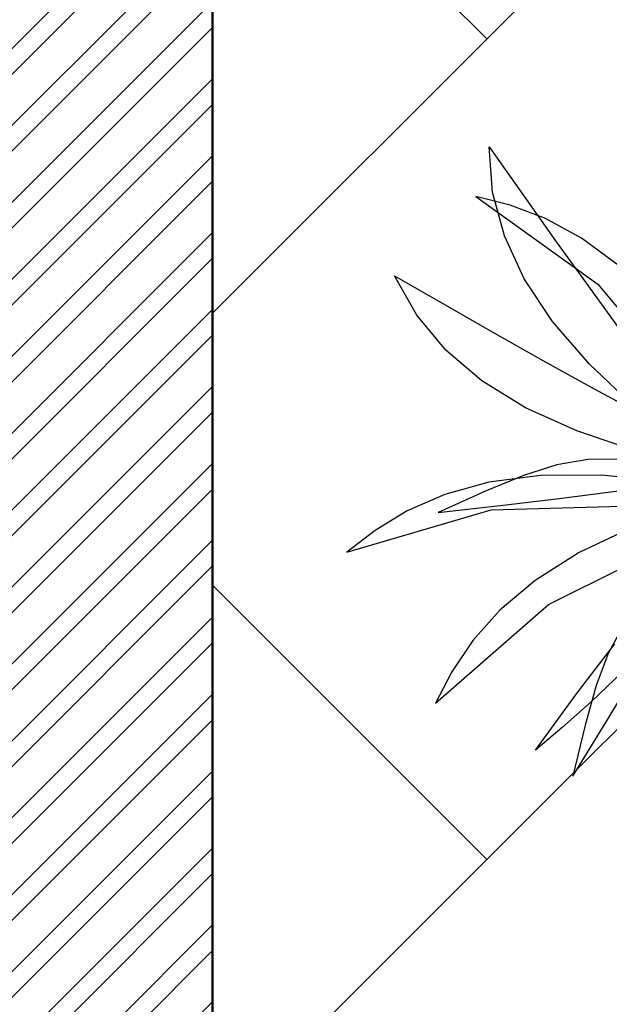
# Model space of a CAD drawing. Units: inches. Extents: x 3590 to 5167, y 65 to 1917.
# Tile 49 of 100: x 4927 to 4947, y 1504 to 1538. Entities that reach past the tile are written whole.
import ezdxf

# ---------------------------------------------------------------- set-up
doc = ezdxf.new("R2010")
doc.units = ezdxf.units.IN
for name, color, linetype, lineweight in [('A-FLOR-PATT', 8, 'Continuous', 13), ('A-WALL', 7, 'Continuous', 50), ('A-WALL-PATT', 251, 'Continuous', 13), ('L-PLNT', 94, 'Continuous', 18)]:
    doc.layers.add(name, color=color, linetype=linetype, lineweight=lineweight)
doc.layers.add('DIENHOA', color=3, linetype='Continuous')

# ---------------------------------------------------------------- blocks, each defined once
blk = doc.blocks.new('Cay03_mb')
at = {"layer": 'DIENHOA'}
for p, q in [((-365.2, 390.3), (-414.4, 402.8)), ((-414.4, 402.8), (-240.2, 277.8)), ((-314.9, 371.3), (-365.2, 390.3)), ((-263.5, 343.5), (-314.9, 371.3)), ((-211.2, 304.6), (-263.5, 343.5)), ((-240.2, 277.8), (-88.4, 94.9)), ((-298.6, 20.1), (-345, 5.4)), ((-254.7, 27.4), (-298.6, 20.1)), ((-208, 27.8), (-254.7, 27.4)), ((-345, 5.4), (-399.6, -17.1)), ((-225.8, -18.9), (-165.8, -11.3)), ((-399.6, -17.1), (-468, -47.9)), ((-375.6, -37.8), (-295.3, -27.9)), ((-295.3, -27.9), (-225.8, -18.9)), ((-468, -47.9), (-375.6, -37.8)), ((-271, -306.6), (-216.3, -235.6)), ((-206.3, -276.5), (-249.6, -317.8)), ((-329.5, -387.1), (-271, -306.6)), ((-249.6, -317.8), (-291, -354.7)), ((-291, -354.7), (-329.5, -387.1))]:
    blk.add_line(p, q, dxfattribs=at)
for points in [[(-395.6, 473.7), (-347.5, 405.6), (-300.6, 339.5), (-254.3, 275.1), (-208.3, 212.3), (-161.9, 150.9), (-114.8, 90.7), (-66.5, 31.6), (-16.4, -26.7)], [(-16.4, -26.7), (-108.3, 38.6), (-186.9, 101.7), (-252.4, 163.5), (-305.1, 224.4), (-345.4, 285.2), (-373.7, 346.6), (-390.4, 409.2), (-395.6, 473.7)], [(-530.5, 289.7), (-458.3, 248.1), (-387.9, 207.8), (-318.9, 168.7), (-250.8, 131.1), (-182.9, 94.8), (-114.9, 59.9), (-46.2, 26.5), (23.7, -5.4)], [(23.7, -5.4), (-87.2, 15.2), (-185, 39.6), (-270.3, 68.2), (-343.7, 101.4), (-405.9, 139.7), (-457.3, 183.5), (-498.7, 233.4), (-530.5, 289.7)], [(-16.4, -26.7), (-134, -4.7), (-235.3, 5.3), (-322, 4.7), (-395.9, -5), (-458.7, -22.3), (-512.3, -45.7), (-558.2, -73.6), (-598.4, -104.7)], [(-471.9, -320.3), (-310.5, -179.3), (-97.7, -73.3), (23.7, -5.4)], [(23.7, -5.4), (-92.3, -34.8), (-188.4, -68.2), (-266.9, -105.1), (-329.9, -144.9), (-379.7, -187), (-418.5, -230.7), (-448.5, -275.3), (-471.9, -320.3)], [(-598.4, -104.7), (-392.7, -44.4), (-155, -37.4), (-16.4, -26.7)], [(-276.2, -424.4), (-227.3, -345.4), (-185.7, -276.1), (-150, -215.7), (-119.1, -163.8), (-91.5, -119.5), (-66, -82.3), (-41.4, -51.6), (-16.4, -26.7)], [(-16.4, -26.7), (-84.9, -86), (-137, -133.1), (-175.8, -173), (-204.3, -210), (-225.5, -249.1), (-242.5, -294.7), (-258.4, -351.6), (-276.2, -424.4)]]:
    blk.add_lwpolyline(points, dxfattribs=at)

msp = doc.modelspace()

# ---------------------------------------------------------------- hatches: boundary and pattern name
at = {"layer": 'A-FLOR-PATT', "transparency": 33554687}
h = msp.add_hatch(dxfattribs=at)
h.set_pattern_fill('AR-HBONE', color=256, scale=0.2)
h.set_pattern_definition([(45, (-588.972, 0), (0, 28.73682), [60.96, -20.32]), (135, (-574.604, 14.368), (3e-15, 28.73682), [60.96, -20.32])])
h.paths.add_polyline_path([(5071.274, 1796.999), (4933.274, 1796.999), (4933.274, 1753.999), (4962.774, 1753.999, -0.414214), (4928.774, 1719.999), (4933.274, 1718.999), (4933.274, 1334.999), (5071.274, 1334.999)])
h.paths.add_polyline_path([(4951.78, 1521.077), (4951.715, 1521.04), (4951.563, 1520.895)], flags=16)
h.paths.add_polyline_path([(4952.267, 1521.376), (4952.198, 1521.371), (4952.198, 1521.356)], flags=0)
h.paths.add_polyline_path([(4967.051, 1529.728), (4965.231, 1528.694), (4963.411, 1527.714), (4961.756, 1526.851), (4963.589, 1527.449), (4964.036, 1527.478), (4962.975, 1527.249), (4961.76, 1526.852), (4959.792, 1525.834), (4958.005, 1524.895), (4956.24, 1523.93), (4954.504, 1522.919), (4954.129, 1522.682), (4953.361, 1521.997), (4953.366, 1521.998), (4953.605, 1522.064), (4955.106, 1522.761), (4956.921, 1523.434), (4958.678, 1523.915), (4960.358, 1524.2), (4961.945, 1524.286), (4964.171, 1524.108), (4965.958, 1523.309), (4963.863, 1522.976), (4965.187, 1522.499), (4963.366, 1522.497), (4961.545, 1522.487), (4959.764, 1522.461), (4958.304, 1522.419), (4957.974, 1522.388), (4956.307, 1522.232), (4954.718, 1522.071), (4953.251, 1521.899), (4953.525, 1521.623), (4954.331, 1521.379), (4956.243, 1521.23), (4958.039, 1520.93), (4959.684, 1520.483), (4961.16, 1519.896), (4963.107, 1518.8), (4964.393, 1517.325), (4962.973, 1517.726), (4964.558, 1516.661), (4965.407, 1515.708), (4963.507, 1516.322), (4961.68, 1517.005), (4959.935, 1517.745), (4958.282, 1518.528), (4956.732, 1519.343), (4955.295, 1520.175), (4954.672, 1520.572), (4954.513, 1520.627), (4955.658, 1519.318), (4956.703, 1517.982), (4957.644, 1516.647), (4958.485, 1515.334), (4959.55, 1513.524), (4960.438, 1511.769), (4958.841, 1513.62), (4957.452, 1515.325), (4955.819, 1517.459), (4956.665, 1515.448), (4957.111, 1513.923), (4957.447, 1511.714), (4957.076, 1509.793), (4956.538, 1511.11), (4955.992, 1512.569), (4955.444, 1514.125), (4954.898, 1515.735), (4954.357, 1517.356), (4953.824, 1518.943), (4953.305, 1520.452), (4953.065, 1521.116), (4952.971, 1521.146), (4952.949, 1521.086), (4952.73, 1520.199), (4953.37, 1518.024), (4953.757, 1516.373), (4954.051, 1514.765), (4954.264, 1513.221), (4954.471, 1511.131), (4954.497, 1510.402), (4954.409, 1511.76), (4954.264, 1513.221), (4954.051, 1514.765), (4953.757, 1516.373), (4953.37, 1518.024), (4952.877, 1519.698), (4952.716, 1520.141), (4952.533, 1519.059), (4952.374, 1517.789), (4952.219, 1516.312), (4952.046, 1514.6), (4951.833, 1512.626), (4951.557, 1510.363), (4951.203, 1512.168), (4950.852, 1514.339), (4950.985, 1516.376), (4951.66, 1518.286), (4952.593, 1520.481), (4952.357, 1521.13), (4951.855, 1520.328), (4950.839, 1518.908), (4949.777, 1517.587), (4948.916, 1516.617), (4948.111, 1515.256), (4947.089, 1513.554), (4945.889, 1511.615), (4946.326, 1513.402), (4946.562, 1514.249), (4945.528, 1513.327), (4944.581, 1512.531), (4946.018, 1514.508), (4947.204, 1516.048), (4947.893, 1517.313), (4949.307, 1518.764), (4950.414, 1519.767), (4950.451, 1519.806), (4952.267, 1521.376), (4951.645, 1521.493), (4950.404, 1521.18), (4948.044, 1520.359), (4946.119, 1519.452), (4944.572, 1518.475), (4943.35, 1517.443), (4941.997, 1515.92), (4941.661, 1515.275), (4942.813, 1516.99), (4944.572, 1518.475), (4946.119, 1519.452), (4948.044, 1520.359), (4950.404, 1521.18), (4951.645, 1521.493), (4949.647, 1521.868), (4948.6, 1521.756), (4947.126, 1521.57), (4945.42, 1521.348), (4943.45, 1521.105), (4941.183, 1520.856), (4942.86, 1521.613), (4943.873, 1522.03), (4942.952, 1521.909), (4941.41, 1521.485), (4939.543, 1520.67), (4938.968, 1520.226), (4940.733, 1521.299), (4942.952, 1521.909), (4943.702, 1522.008), (4945.894, 1522.7), (4947.565, 1522.714), (4948.921, 1522.566), (4951.131, 1522.183), (4950.971, 1522.297), (4948.129, 1523.006), (4946.035, 1523.707), (4944.232, 1524.521), (4942.707, 1525.461), (4941.444, 1526.537), (4940.43, 1527.761), (4939.649, 1529.143), (4941.421, 1528.122), (4943.147, 1527.132), (4944.841, 1526.175), (4946.514, 1525.25), (4948.179, 1524.359), (4948.365, 1524.263), (4946.475, 1526.045), (4945.181, 1527.54), (4944.19, 1529.033), (4943.496, 1530.54), (4943.278, 1531.36), (4942.498, 1531.919), (4943.114, 1531.762), (4942.959, 1533.659), (4944.14, 1531.989), (4944.612, 1531.323), (4946.202, 1530.463), (4947.486, 1529.509), (4948.79, 1528.226), (4950.368, 1526.237), (4949.485, 1528.155), (4948.851, 1530.123), (4948.491, 1532.041), (4948.381, 1533.918), (4948.501, 1535.76), (4948.827, 1537.573), (4949.418, 1535.565), (4949.957, 1533.569), (4950.464, 1531.586), (4950.961, 1529.617), (4951.391, 1527.954), (4951.724, 1530.687), (4952.201, 1532.58), (4952.889, 1534.33), (4953.77, 1535.951), (4954.827, 1537.46), (4954.521, 1535.39), (4954.273, 1533.937), (4955.58, 1535.663), (4956.748, 1536.739), (4956.159, 1534.78), (4955.589, 1532.873), (4955.043, 1531.006), (4954.525, 1529.166), (4954.038, 1527.341), (4953.638, 1525.733), (4953.611, 1525.586), (4953.398, 1524.166), (4953.382, 1524.009), (4954.07, 1525.476), (4954.912, 1527.022), (4956.136, 1528.894), (4957.847, 1530.577), (4959.376, 1531.54), (4958.256, 1530.104), (4957.143, 1528.663), (4956.066, 1527.243), (4955.056, 1525.871), (4954.141, 1524.571), (4953.352, 1523.372), (4953.311, 1523.303), (4953.273, 1522.925), (4953.261, 1522.382), (4954.103, 1523.373), (4954.63, 1524.284), (4955.961, 1526.358), (4957.23, 1528.13), (4958.421, 1529.609), (4960.037, 1531.368), (4961.374, 1532.375), (4962.101, 1532.77), (4961.07, 1531.061), (4959.987, 1529.438), (4958.869, 1527.908), (4958.15, 1527.007), (4959.803, 1528.003), (4961.589, 1528.793), (4963.391, 1529.328), (4965.211, 1529.632)], flags=16)
h.paths.add_polyline_path([(4962.944, 1523.182), (4961.107, 1523.422), (4960.392, 1523.362), (4962.35, 1523.331)], flags=0)
h.paths.add_polyline_path([(5049.541, 1584.551), (5049.476, 1584.515), (5049.325, 1584.37)], flags=16)
h.paths.add_polyline_path([(5050.028, 1584.851), (5049.959, 1584.845), (5049.959, 1584.83)], flags=0)
h.paths.add_polyline_path([(5042.333, 1581.949), (5043.88, 1582.926), (5045.806, 1583.833), (5048.165, 1584.654), (5049.406, 1584.967), (5047.408, 1585.342), (5046.361, 1585.231), (5044.888, 1585.044), (5043.181, 1584.822), (5041.211, 1584.579), (5038.944, 1584.33), (5040.622, 1585.087), (5041.634, 1585.504), (5040.713, 1585.383), (5039.171, 1584.959), (5037.304, 1584.144), (5036.729, 1583.7), (5038.494, 1584.773), (5040.713, 1585.383), (5041.463, 1585.482), (5043.655, 1586.174), (5045.326, 1586.188), (5046.682, 1586.04), (5048.893, 1585.657), (5048.732, 1585.771), (5045.891, 1586.48), (5043.796, 1587.181), (5041.994, 1587.996), (5040.468, 1588.935), (5039.205, 1590.011), (5038.191, 1591.235), (5037.41, 1592.617), (5039.182, 1591.596), (5040.909, 1590.607), (5042.602, 1589.649), (5044.275, 1588.724), (5045.94, 1587.833), (5046.126, 1587.738), (5044.237, 1589.519), (5042.942, 1591.015), (5041.952, 1592.508), (5041.257, 1594.014), (5041.039, 1594.834), (5040.26, 1595.393), (5040.875, 1595.237), (5040.721, 1597.133), (5041.901, 1595.463), (5042.373, 1594.798), (5043.963, 1593.938), (5045.247, 1592.983), (5046.552, 1591.701), (5048.129, 1589.712), (5047.247, 1591.63), (5046.613, 1593.597), (5046.252, 1595.515), (5046.142, 1597.392), (5046.262, 1599.234), (5046.588, 1601.047), (5047.179, 1599.039), (5047.718, 1597.043), (5048.225, 1595.06), (5048.722, 1593.091), (5049.152, 1591.429), (5049.485, 1594.161), (5049.962, 1596.054), (5050.65, 1597.804), (5051.532, 1599.425), (5052.589, 1600.934), (5052.283, 1598.864), (5052.034, 1597.411), (5053.341, 1599.137), (5054.509, 1600.213), (5053.92, 1598.254), (5053.35, 1596.348), (5052.805, 1594.48), (5052.286, 1592.64), (5051.799, 1590.815), (5051.4, 1589.207), (5051.373, 1589.06), (5051.159, 1587.64), (5051.143, 1587.483), (5051.831, 1588.95), (5052.673, 1590.496), (5053.898, 1592.368), (5055.608, 1594.051), (5057.137, 1595.014), (5056.017, 1593.578), (5054.904, 1592.137), (5053.828, 1590.717), (5052.817, 1589.345), (5051.902, 1588.046), (5051.113, 1586.846), (5051.072, 1586.777), (5051.034, 1586.399), (5051.022, 1585.856), (5051.864, 1586.847), (5052.391, 1587.758), (5053.723, 1589.832), (5054.991, 1591.604), (5056.182, 1593.083), (5057.798, 1594.842), (5059.135, 1595.849), (5059.863, 1596.244), (5058.831, 1594.535), (5057.749, 1592.912), (5056.63, 1591.382), (5055.912, 1590.482), (5057.564, 1591.477), (5059.35, 1592.267), (5061.152, 1592.802), (5062.972, 1593.106), (5064.812, 1593.203), (5062.992, 1592.169), (5061.172, 1591.188), (5059.518, 1590.325), (5061.35, 1590.924), (5061.797, 1590.952), (5060.737, 1590.723), (5059.521, 1590.326), (5057.553, 1589.308), (5055.766, 1588.369), (5054.002, 1587.404), (5052.265, 1586.393), (5051.891, 1586.156), (5051.122, 1585.471), (5051.127, 1585.472), (5051.366, 1585.538), (5052.867, 1586.235), (5054.682, 1586.908), (5056.439, 1587.389), (5058.12, 1587.675), (5059.706, 1587.76), (5061.933, 1587.583), (5063.719, 1586.783), (5061.624, 1586.45), (5062.949, 1585.973), (5061.127, 1585.971), (5059.307, 1585.961), (5057.525, 1585.935), (5056.065, 1585.893), (5055.735, 1585.862), (5054.068, 1585.707), (5052.479, 1585.546), (5051.012, 1585.373), (5051.286, 1585.097), (5052.092, 1584.853), (5054.004, 1584.704), (5055.8, 1584.404), (5057.446, 1583.958), (5058.921, 1583.37), (5060.868, 1582.274), (5062.154, 1580.799), (5060.734, 1581.2), (5062.32, 1580.135), (5063.168, 1579.182), (5061.269, 1579.796), (5059.441, 1580.479), (5057.696, 1581.219), (5056.043, 1582.003), (5054.493, 1582.817), (5053.057, 1583.649), (5052.433, 1584.047), (5052.274, 1584.101), (5053.42, 1582.793), (5054.464, 1581.457), (5055.405, 1580.121), (5056.247, 1578.809), (5057.311, 1576.998), (5058.199, 1575.244), (5056.602, 1577.094), (5055.213, 1578.799), (5053.58, 1580.933), (5054.427, 1578.922), (5054.872, 1577.397), (5055.208, 1575.189), (5054.838, 1573.267), (5054.299, 1574.584), (5053.754, 1576.043), (5053.206, 1577.599), (5052.659, 1579.209), (5052.118, 1580.83), (5051.585, 1582.417), (5051.066, 1583.927), (5050.826, 1584.59), (5050.733, 1584.62), (5050.711, 1584.561), (5050.491, 1583.673), (5051.131, 1581.498), (5051.518, 1579.847), (5051.813, 1578.24), (5052.026, 1576.695), (5052.233, 1574.605), (5052.258, 1573.876), (5052.17, 1575.234), (5052.026, 1576.695), (5051.813, 1578.24), (5051.518, 1579.847), (5051.131, 1581.498), (5050.638, 1583.172), (5050.477, 1583.615), (5050.294, 1582.533), (5050.136, 1581.263), (5049.981, 1579.786), (5049.807, 1578.074), (5049.594, 1576.1), (5049.318, 1573.837), (5048.965, 1575.642), (5048.613, 1577.813), (5048.747, 1579.85), (5049.421, 1581.76), (5050.354, 1583.955), (5050.118, 1584.604), (5049.616, 1583.802), (5048.6, 1582.382), (5047.538, 1581.061), (5046.677, 1580.091), (5045.872, 1578.73), (5044.85, 1577.028), (5043.651, 1575.089), (5044.087, 1576.877), (5044.324, 1577.723), (5043.289, 1576.801), (5042.342, 1576.005), (5043.779, 1577.982), (5044.966, 1579.522), (5045.655, 1580.787), (5047.068, 1582.239), (5048.175, 1583.241), (5048.213, 1583.28), (5050.028, 1584.851), (5049.406, 1584.967), (5048.165, 1584.654), (5045.806, 1583.833), (5043.88, 1582.926), (5042.333, 1581.949), (5041.111, 1580.917), (5039.758, 1579.394), (5039.423, 1578.749), (5040.575, 1580.464)], flags=16)
h.paths.add_polyline_path([(4954.799, 1533.12), (4954.262, 1532.079), (4953.831, 1530.935), (4953.505, 1529.636), (4953.283, 1528.133), (4953.167, 1526.376), (4953.156, 1524.315), (4953.277, 1521.236), (4952.802, 1521.842), (4951.557, 1521.998), (4950.976, 1521.961), (4952.661, 1521.941), (4952.802, 1521.842), (4953.152, 1523.593), (4953.167, 1526.376), (4953.283, 1528.133), (4953.609, 1530.346), (4954.456, 1532.592)], flags=0)
h.paths.add_polyline_path([(5050.563, 1585.316), (5049.318, 1585.472), (5048.737, 1585.435), (5050.422, 1585.415), (5050.563, 1585.316), (5050.914, 1587.067), (5050.928, 1589.851), (5051.045, 1591.607), (5051.371, 1593.82), (5052.217, 1596.066), (5052.56, 1596.594), (5052.024, 1595.554), (5051.592, 1594.409), (5051.266, 1593.11), (5051.045, 1591.607), (5050.928, 1589.851), (5050.918, 1587.789), (5051.038, 1584.71)], flags=0)
h.paths.add_polyline_path([(5058.153, 1586.836), (5060.111, 1586.805), (5060.705, 1586.656), (5058.868, 1586.896)], flags=0)
h.paths.add_polyline_path([(5049.541, 1430.936), (5049.476, 1430.9), (5049.325, 1430.755)], flags=16)
h.paths.add_polyline_path([(5050.028, 1431.236), (5049.959, 1431.231), (5049.959, 1431.215)], flags=0)
h.paths.add_polyline_path([(5046.588, 1447.432), (5047.179, 1445.425), (5047.718, 1443.429), (5048.225, 1441.446), (5048.722, 1439.476), (5049.152, 1437.814), (5049.485, 1440.546), (5049.962, 1442.439), (5050.65, 1444.189), (5051.532, 1445.811), (5052.589, 1447.319), (5052.283, 1445.249), (5052.034, 1443.796), (5053.341, 1445.522), (5054.509, 1446.598), (5053.92, 1444.64), (5053.35, 1442.733), (5052.805, 1440.865), (5052.286, 1439.025), (5051.799, 1437.201), (5051.4, 1435.592), (5051.373, 1435.445), (5051.159, 1434.025), (5051.143, 1433.868), (5051.831, 1435.335), (5052.673, 1436.881), (5053.898, 1438.753), (5055.608, 1440.436), (5057.137, 1441.4), (5056.017, 1439.963), (5054.904, 1438.522), (5053.828, 1437.102), (5052.817, 1435.73), (5051.902, 1434.431), (5051.113, 1433.231), (5051.072, 1433.162), (5051.034, 1432.784), (5051.022, 1432.242), (5051.864, 1433.232), (5052.391, 1434.143), (5053.723, 1436.217), (5054.991, 1437.989), (5056.182, 1439.468), (5057.798, 1441.227), (5059.135, 1442.235), (5059.863, 1442.629), (5058.831, 1440.921), (5057.749, 1439.298), (5056.63, 1437.767), (5055.912, 1436.867), (5057.564, 1437.863), (5059.35, 1438.652), (5061.152, 1439.187), (5062.972, 1439.491), (5064.812, 1439.588), (5062.992, 1438.554), (5061.172, 1437.573), (5059.518, 1436.71), (5061.35, 1437.309), (5061.797, 1437.337), (5060.737, 1437.108), (5059.521, 1436.711), (5057.553, 1435.693), (5055.766, 1434.754), (5054.002, 1433.789), (5052.265, 1432.778), (5051.891, 1432.541), (5051.122, 1431.856), (5051.127, 1431.857), (5051.366, 1431.923), (5052.867, 1432.62), (5054.682, 1433.293), (5056.439, 1433.775), (5058.12, 1434.06), (5059.706, 1434.145), (5061.933, 1433.968), (5063.719, 1433.168), (5061.624, 1432.835), (5062.949, 1432.358), (5061.127, 1432.357), (5059.307, 1432.346), (5057.525, 1432.32), (5056.065, 1432.278), (5055.735, 1432.248), (5054.068, 1432.092), (5052.479, 1431.931), (5051.012, 1431.759), (5051.286, 1431.482), (5052.092, 1431.238), (5054.004, 1431.089), (5055.8, 1430.789), (5057.446, 1430.343), (5058.921, 1429.755), (5060.868, 1428.66), (5062.154, 1427.185), (5060.734, 1427.585), (5062.32, 1426.52), (5063.168, 1425.567), (5061.269, 1426.181), (5059.441, 1426.865), (5057.696, 1427.604), (5056.043, 1428.388), (5054.493, 1429.202), (5053.057, 1430.034), (5052.433, 1430.432), (5052.274, 1430.487), (5053.42, 1429.178), (5054.464, 1427.842), (5055.405, 1426.506), (5056.247, 1425.194), (5057.311, 1423.383), (5058.199, 1421.629), (5056.602, 1423.479), (5055.213, 1425.184), (5053.58, 1427.318), (5054.427, 1425.307), (5054.872, 1423.782), (5055.208, 1421.574), (5054.838, 1419.652), (5054.299, 1420.97), (5053.754, 1422.428), (5053.206, 1423.984), (5052.659, 1425.595), (5052.118, 1427.215), (5051.585, 1428.802), (5051.066, 1430.312), (5050.826, 1430.975), (5050.733, 1431.005), (5050.711, 1430.946), (5050.491, 1430.058), (5051.131, 1427.883), (5051.518, 1426.232), (5051.813, 1424.625), (5052.026, 1423.081), (5052.233, 1420.991), (5052.258, 1420.261), (5052.17, 1421.619), (5052.026, 1423.081), (5051.813, 1424.625), (5051.518, 1426.232), (5051.131, 1427.883), (5050.638, 1429.558), (5050.477, 1430.001), (5050.294, 1428.918), (5050.136, 1427.648), (5049.981, 1426.171), (5049.807, 1424.459), (5049.594, 1422.485), (5049.318, 1420.222), (5048.965, 1422.028), (5048.613, 1424.199), (5048.747, 1426.235), (5049.421, 1428.146), (5050.354, 1430.34), (5050.118, 1430.989), (5049.616, 1430.187), (5048.6, 1428.768), (5047.538, 1427.446), (5046.677, 1426.477), (5045.872, 1425.116), (5044.85, 1423.413), (5043.651, 1421.474), (5044.087, 1423.262), (5044.324, 1424.109), (5043.289, 1423.186), (5042.342, 1422.391), (5043.779, 1424.368), (5044.966, 1425.907), (5045.655, 1427.173), (5047.068, 1428.624), (5048.175, 1429.627), (5048.213, 1429.666), (5050.028, 1431.236), (5049.406, 1431.353), (5048.165, 1431.039), (5045.806, 1430.218), (5043.88, 1429.311), (5042.333, 1428.334), (5041.111, 1427.302), (5039.758, 1425.779), (5039.423, 1425.134), (5040.575, 1426.849), (5042.333, 1428.334), (5043.88, 1429.311), (5045.806, 1430.218), (5048.165, 1431.039), (5049.406, 1431.353), (5047.408, 1431.727), (5046.361, 1431.616), (5044.888, 1431.429), (5043.181, 1431.207), (5041.211, 1430.964), (5038.944, 1430.715), (5040.622, 1431.472), (5041.634, 1431.89), (5040.713, 1431.769), (5039.171, 1431.345), (5037.304, 1430.53), (5036.729, 1430.085), (5038.494, 1431.158), (5040.713, 1431.769), (5041.463, 1431.867), (5043.655, 1432.559), (5045.326, 1432.573), (5046.682, 1432.425), (5048.893, 1432.042), (5048.732, 1432.156), (5045.891, 1432.865), (5043.796, 1433.566), (5041.994, 1434.381), (5040.468, 1435.321), (5039.205, 1436.396), (5038.191, 1437.62), (5037.41, 1439.002), (5039.182, 1437.982), (5040.909, 1436.992), (5042.602, 1436.034), (5044.275, 1435.109), (5045.94, 1434.218), (5046.126, 1434.123), (5044.237, 1435.904), (5042.942, 1437.4), (5041.952, 1438.893), (5041.257, 1440.399), (5041.039, 1441.219), (5040.26, 1441.778), (5040.875, 1441.622), (5040.721, 1443.518), (5041.901, 1441.848), (5042.373, 1441.183), (5043.963, 1440.323), (5045.247, 1439.369), (5046.552, 1438.086), (5048.129, 1436.097), (5047.247, 1438.015), (5046.613, 1439.982), (5046.252, 1441.901), (5046.142, 1443.778), (5046.262, 1445.619)], flags=16)
h.paths.add_polyline_path([(5052.382, 1444.255), (5051.623, 1442.78), (5052.024, 1441.939), (5052.56, 1442.98)], flags=0)
h.paths.add_polyline_path([(5050.563, 1431.701), (5049.318, 1431.857), (5048.737, 1431.821), (5050.422, 1431.8)], flags=0)
h.paths.add_polyline_path([(5058.153, 1433.221), (5060.111, 1433.19), (5060.705, 1433.041), (5058.868, 1433.281)], flags=0)
h.paths.add_polyline_path([(5049.541, 1352.285), (5049.476, 1352.249), (5049.325, 1352.104)], flags=16)
h.paths.add_polyline_path([(5050.028, 1352.585), (5049.959, 1352.58), (5049.959, 1352.564)], flags=0)
h.paths.add_polyline_path([(5046.588, 1368.781), (5047.179, 1366.774), (5047.718, 1364.778), (5048.225, 1362.795), (5048.722, 1360.825), (5049.152, 1359.163), (5049.485, 1361.896), (5049.962, 1363.789), (5050.65, 1365.538), (5051.532, 1367.16), (5052.589, 1368.669), (5052.283, 1366.598), (5052.034, 1365.145), (5053.341, 1366.871), (5054.509, 1367.947), (5053.92, 1365.989), (5053.35, 1364.082), (5052.805, 1362.214), (5052.286, 1360.374), (5051.799, 1358.55), (5051.4, 1356.942), (5051.373, 1356.794), (5051.159, 1355.374), (5051.143, 1355.218), (5051.831, 1356.684), (5052.673, 1358.23), (5053.898, 1360.102), (5055.608, 1361.786), (5057.137, 1362.749), (5056.017, 1361.313), (5054.904, 1359.872), (5053.828, 1358.452), (5052.817, 1357.079), (5051.902, 1355.78), (5051.113, 1354.581), (5051.072, 1354.512), (5051.034, 1354.133), (5051.022, 1353.591), (5051.864, 1354.581), (5052.391, 1355.492), (5053.723, 1357.566), (5054.991, 1359.338), (5056.182, 1360.817), (5057.798, 1362.577), (5059.135, 1363.584), (5059.863, 1363.979), (5058.831, 1362.27), (5057.749, 1360.647), (5056.63, 1359.117), (5055.912, 1358.216), (5057.564, 1359.212), (5059.35, 1360.001), (5061.152, 1360.536), (5062.972, 1360.841), (5064.812, 1360.937), (5062.992, 1359.903), (5061.172, 1358.923), (5059.518, 1358.059), (5061.35, 1358.658), (5061.797, 1358.687), (5060.737, 1358.458), (5059.521, 1358.061), (5057.553, 1357.043), (5055.766, 1356.103), (5054.002, 1355.138), (5052.265, 1354.127), (5051.891, 1353.89), (5051.122, 1353.206), (5051.127, 1353.206), (5051.366, 1353.272), (5052.867, 1353.969), (5054.682, 1354.643), (5056.439, 1355.124), (5058.12, 1355.409), (5059.706, 1355.495), (5061.933, 1355.317), (5063.719, 1354.518), (5061.624, 1354.184), (5062.949, 1353.708), (5061.127, 1353.706), (5059.307, 1353.695), (5057.525, 1353.669), (5056.065, 1353.627), (5055.735, 1353.597), (5054.068, 1353.441), (5052.479, 1353.28), (5051.012, 1353.108), (5051.286, 1352.831), (5052.092, 1352.587), (5054.004, 1352.439), (5055.8, 1352.138), (5057.446, 1351.692), (5058.921, 1351.104), (5060.868, 1350.009), (5062.154, 1348.534), (5060.734, 1348.935), (5062.32, 1347.869), (5063.168, 1346.916), (5061.269, 1347.53), (5059.441, 1348.214), (5057.696, 1348.954), (5056.043, 1349.737), (5054.493, 1350.551), (5053.057, 1351.383), (5052.433, 1351.781), (5052.274, 1351.836), (5053.42, 1350.527), (5054.464, 1349.191), (5055.405, 1347.855), (5056.247, 1346.543), (5057.311, 1344.733), (5058.199, 1342.978), (5056.602, 1344.828), (5055.213, 1346.534), (5053.58, 1348.667), (5054.427, 1346.656), (5054.872, 1345.132), (5055.208, 1342.923), (5054.838, 1341.002), (5054.299, 1342.319), (5053.754, 1343.778), (5053.206, 1345.334), (5052.659, 1346.944), (5052.118, 1348.564), (5051.585, 1350.151), (5051.066, 1351.661), (5050.826, 1352.324), (5050.733, 1352.355), (5050.711, 1352.295), (5050.491, 1351.408), (5051.131, 1349.232), (5051.518, 1347.581), (5051.813, 1345.974), (5052.026, 1344.43), (5052.233, 1342.34), (5052.258, 1341.61), (5052.17, 1342.969), (5052.026, 1344.43), (5051.813, 1345.974), (5051.518, 1347.581), (5051.131, 1349.232), (5050.638, 1350.907), (5050.477, 1351.35), (5050.294, 1350.267), (5050.136, 1348.997), (5049.981, 1347.52), (5049.807, 1345.809), (5049.594, 1343.835), (5049.318, 1341.571), (5048.965, 1343.377), (5048.613, 1345.548), (5048.747, 1347.585), (5049.421, 1349.495), (5050.354, 1351.689), (5050.118, 1352.339), (5049.616, 1351.536), (5048.6, 1350.117), (5047.538, 1348.795), (5046.677, 1347.826), (5045.872, 1346.465), (5044.85, 1344.763), (5043.651, 1342.824), (5044.087, 1344.611), (5044.324, 1345.458), (5043.289, 1344.535), (5042.342, 1343.74), (5043.779, 1345.717), (5044.966, 1347.256), (5045.655, 1348.522), (5047.068, 1349.973), (5048.175, 1350.976), (5048.213, 1351.015), (5050.028, 1352.585), (5049.406, 1352.702), (5048.165, 1352.388), (5045.806, 1351.567), (5043.88, 1350.661), (5042.333, 1349.683), (5041.111, 1348.651), (5039.758, 1347.128), (5039.423, 1346.483), (5040.575, 1348.198), (5042.333, 1349.683), (5043.88, 1350.661), (5045.806, 1351.567), (5048.165, 1352.388), (5049.406, 1352.702), (5047.408, 1353.076), (5046.361, 1352.965), (5044.888, 1352.779), (5043.181, 1352.556), (5041.211, 1352.313), (5038.944, 1352.065), (5040.622, 1352.821), (5041.634, 1353.239), (5040.713, 1353.118), (5039.171, 1352.694), (5037.304, 1351.879), (5036.729, 1351.434), (5038.494, 1352.508), (5040.713, 1353.118), (5041.463, 1353.216), (5043.655, 1353.909), (5045.326, 1353.923), (5046.682, 1353.774), (5048.893, 1353.391), (5048.732, 1353.506), (5045.891, 1354.214), (5043.796, 1354.915), (5041.994, 1355.73), (5040.468, 1356.67), (5039.205, 1357.746), (5038.191, 1358.969), (5037.41, 1360.352), (5039.182, 1359.331), (5040.909, 1358.341), (5042.602, 1357.383), (5044.275, 1356.458), (5045.94, 1355.567), (5046.126, 1355.472), (5044.237, 1357.253), (5042.942, 1358.749), (5041.952, 1360.242), (5041.257, 1361.748), (5041.039, 1362.568), (5040.26, 1363.128), (5040.875, 1362.971), (5040.721, 1364.867), (5041.901, 1363.197), (5042.373, 1362.532), (5043.963, 1361.672), (5045.247, 1360.718), (5046.552, 1359.435), (5048.129, 1357.446), (5047.247, 1359.364), (5046.613, 1361.331), (5046.252, 1363.25), (5046.142, 1365.127), (5046.262, 1366.969)], flags=16)
h.paths.add_polyline_path([(5052.382, 1365.604), (5051.623, 1364.129), (5052.024, 1363.288), (5052.56, 1364.329)], flags=0)
h.paths.add_polyline_path([(4951.78, 1698.041), (4951.715, 1698.005), (4951.563, 1697.859)], flags=16)
h.paths.add_polyline_path([(4952.267, 1698.341), (4952.198, 1698.335), (4952.198, 1698.32)], flags=0)
h.paths.add_polyline_path([(4957.076, 1686.757), (4956.538, 1688.074), (4955.992, 1689.533), (4955.444, 1691.089), (4954.898, 1692.699), (4954.357, 1694.32), (4953.824, 1695.907), (4953.305, 1697.417), (4953.065, 1698.08), (4952.971, 1698.11), (4952.949, 1698.051), (4952.73, 1697.163), (4953.37, 1694.988), (4953.757, 1693.337), (4954.051, 1691.729), (4954.264, 1690.185), (4954.471, 1688.095), (4954.497, 1687.366), (4954.409, 1688.724), (4954.264, 1690.185), (4954.051, 1691.729), (4953.757, 1693.337), (4953.37, 1694.988), (4952.877, 1696.662), (4952.716, 1697.105), (4952.533, 1696.023), (4952.374, 1694.753), (4952.219, 1693.276), (4952.046, 1691.564), (4951.833, 1689.59), (4951.557, 1687.327), (4951.203, 1689.132), (4950.852, 1691.303), (4950.985, 1693.34), (4951.66, 1695.25), (4952.593, 1697.445), (4952.357, 1698.094), (4951.855, 1697.292), (4950.839, 1695.872), (4949.777, 1694.551), (4948.916, 1693.581), (4948.111, 1692.22), (4947.089, 1690.518), (4945.889, 1688.579), (4946.326, 1690.366), (4946.562, 1691.213), (4945.528, 1690.291), (4944.581, 1689.495), (4946.018, 1691.472), (4947.204, 1693.012), (4947.893, 1694.277), (4949.307, 1695.729), (4950.414, 1696.731), (4950.451, 1696.77), (4952.267, 1698.341), (4951.645, 1698.457), (4950.404, 1698.144), (4948.044, 1697.323), (4946.119, 1696.416), (4944.572, 1695.439), (4943.35, 1694.407), (4941.997, 1692.884), (4941.661, 1692.239), (4942.813, 1693.954), (4944.572, 1695.439), (4946.119, 1696.416), (4948.044, 1697.323), (4950.404, 1698.144), (4951.645, 1698.457), (4949.647, 1698.832), (4948.6, 1698.72), (4947.126, 1698.534), (4945.42, 1698.312), (4943.45, 1698.069), (4941.183, 1697.82), (4942.86, 1698.577), (4943.873, 1698.994), (4942.952, 1698.873), (4941.41, 1698.449), (4939.543, 1697.634), (4938.968, 1697.19), (4940.733, 1698.263), (4942.952, 1698.873), (4943.702, 1698.972), (4945.894, 1699.664), (4947.565, 1699.678), (4948.921, 1699.53), (4951.131, 1699.147), (4950.971, 1699.261), (4948.129, 1699.97), (4946.035, 1700.671), (4944.232, 1701.486), (4942.707, 1702.425), (4941.444, 1703.501), (4940.43, 1704.725), (4939.649, 1706.107), (4941.421, 1705.086), (4943.147, 1704.097), (4944.841, 1703.139), (4946.514, 1702.214), (4948.179, 1701.323), (4948.365, 1701.227), (4946.475, 1703.009), (4945.181, 1704.505), (4944.19, 1705.997), (4943.496, 1707.504), (4943.278, 1708.324), (4942.498, 1708.883), (4943.114, 1708.727), (4942.959, 1710.623), (4944.14, 1708.953), (4944.612, 1708.287), (4946.202, 1707.428), (4947.486, 1706.473), (4948.79, 1705.191), (4950.368, 1703.202), (4949.485, 1705.12), (4948.851, 1707.087), (4948.491, 1709.005), (4948.381, 1710.882), (4948.501, 1712.724), (4948.827, 1714.537), (4949.418, 1712.529), (4949.957, 1710.533), (4950.464, 1708.55), (4950.961, 1706.581), (4951.391, 1704.919), (4951.724, 1707.651), (4952.201, 1709.544), (4952.889, 1711.294), (4953.77, 1712.915), (4954.827, 1714.424), (4954.521, 1712.354), (4954.273, 1710.901), (4955.58, 1712.627), (4956.748, 1713.703), (4956.159, 1711.744), (4955.589, 1709.837), (4955.043, 1707.97), (4954.525, 1706.13), (4954.038, 1704.305), (4953.638, 1702.697), (4953.611, 1702.55), (4953.398, 1701.13), (4953.382, 1700.973), (4954.07, 1702.44), (4954.912, 1703.986), (4956.136, 1705.858), (4957.847, 1707.541), (4959.376, 1708.504), (4958.256, 1707.068), (4957.143, 1705.627), (4956.066, 1704.207), (4955.056, 1702.835), (4954.141, 1701.536), (4953.352, 1700.336), (4953.311, 1700.267), (4953.273, 1699.889), (4953.261, 1699.346), (4954.103, 1700.337), (4954.63, 1701.248), (4955.961, 1703.322), (4957.23, 1705.094), (4958.421, 1706.573), (4960.037, 1708.332), (4961.374, 1709.339), (4962.101, 1709.734), (4961.07, 1708.025), (4959.987, 1706.402), (4958.869, 1704.872), (4958.15, 1703.972), (4959.803, 1704.967), (4961.589, 1705.757), (4963.391, 1706.292), (4965.211, 1706.596), (4967.051, 1706.692), (4965.231, 1705.659), (4963.411, 1704.678), (4961.756, 1703.815), (4963.589, 1704.413), (4964.036, 1704.442), (4962.975, 1704.213), (4961.76, 1703.816), (4959.792, 1702.798), (4958.005, 1701.859), (4956.24, 1700.894), (4954.504, 1699.883), (4954.129, 1699.646), (4953.361, 1698.961), (4953.366, 1698.962), (4953.605, 1699.028), (4955.106, 1699.725), (4956.921, 1700.398), (4958.678, 1700.879), (4960.358, 1701.164), (4961.945, 1701.25), (4964.171, 1701.073), (4965.958, 1700.273), (4963.863, 1699.94), (4965.187, 1699.463), (4963.366, 1699.461), (4961.545, 1699.451), (4959.764, 1699.425), (4958.304, 1699.383), (4957.974, 1699.352), (4956.307, 1699.197), (4954.718, 1699.036), (4953.251, 1698.863), (4953.525, 1698.587), (4954.331, 1698.343), (4956.243, 1698.194), (4958.039, 1697.894), (4959.684, 1697.447), (4961.16, 1696.86), (4963.107, 1695.764), (4964.393, 1694.289), (4962.973, 1694.69), (4964.558, 1693.625), (4965.407, 1692.672), (4963.507, 1693.286), (4961.68, 1693.969), (4959.935, 1694.709), (4958.282, 1695.492), (4956.732, 1696.307), (4955.295, 1697.139), (4954.672, 1697.536), (4954.513, 1697.591), (4955.658, 1696.282), (4956.703, 1694.946), (4957.644, 1693.611), (4958.485, 1692.298), (4959.55, 1690.488), (4960.438, 1688.733), (4958.841, 1690.584), (4957.452, 1692.289), (4955.819, 1694.423), (4956.665, 1692.412), (4957.111, 1690.887), (4957.447, 1688.678)], flags=16)
h.paths.add_polyline_path([(5050.563, 1353.05), (5049.318, 1353.207), (5048.737, 1353.17), (5050.422, 1353.15)], flags=0)
h.paths.add_polyline_path([(4951.78, 1351.486), (4951.715, 1351.45), (4951.563, 1351.305)], flags=16)
h.paths.add_polyline_path([(4952.267, 1351.786), (4952.198, 1351.78), (4952.198, 1351.765)], flags=0)
h.paths.add_polyline_path([(4954.827, 1367.869), (4954.521, 1365.799), (4954.273, 1364.346), (4955.58, 1366.072), (4956.748, 1367.148), (4956.159, 1365.19), (4955.589, 1363.283), (4955.043, 1361.415), (4954.525, 1359.575), (4954.038, 1357.751), (4953.638, 1356.142), (4953.611, 1355.995), (4953.398, 1354.575), (4953.382, 1354.418), (4954.07, 1355.885), (4954.912, 1357.431), (4956.136, 1359.303), (4957.847, 1360.986), (4959.376, 1361.95), (4958.256, 1360.513), (4957.143, 1359.072), (4956.066, 1357.652), (4955.056, 1356.28), (4954.141, 1354.981), (4953.352, 1353.781), (4953.311, 1353.712), (4953.273, 1353.334), (4953.261, 1352.792), (4954.103, 1353.782), (4954.63, 1354.693), (4955.961, 1356.767), (4957.23, 1358.539), (4958.421, 1360.018), (4960.037, 1361.777), (4961.374, 1362.785), (4962.101, 1363.179), (4961.07, 1361.471), (4959.987, 1359.848), (4958.869, 1358.317), (4958.15, 1357.417), (4959.803, 1358.413), (4961.589, 1359.202), (4963.391, 1359.737), (4965.211, 1360.041), (4967.051, 1360.138), (4965.231, 1359.104), (4963.411, 1358.123), (4961.756, 1357.26), (4963.589, 1357.859), (4964.036, 1357.887), (4962.975, 1357.658), (4961.76, 1357.261), (4959.792, 1356.243), (4958.005, 1355.304), (4956.24, 1354.339), (4954.504, 1353.328), (4954.129, 1353.091), (4953.361, 1352.406), (4953.366, 1352.407), (4953.605, 1352.473), (4955.106, 1353.17), (4956.921, 1353.843), (4958.678, 1354.325), (4960.358, 1354.61), (4961.945, 1354.695), (4964.171, 1354.518), (4965.958, 1353.718), (4963.863, 1353.385), (4965.187, 1352.908), (4963.366, 1352.907), (4961.545, 1352.896), (4959.764, 1352.87), (4958.304, 1352.828), (4957.974, 1352.798), (4956.307, 1352.642), (4954.718, 1352.481), (4953.251, 1352.309), (4953.525, 1352.032), (4954.331, 1351.788), (4956.243, 1351.639), (4958.039, 1351.339), (4959.684, 1350.893), (4961.16, 1350.305), (4963.107, 1349.21), (4964.393, 1347.735), (4962.973, 1348.135), (4964.558, 1347.07), (4965.407, 1346.117), (4963.507, 1346.731), (4961.68, 1347.414), (4959.935, 1348.154), (4958.282, 1348.938), (4956.732, 1349.752), (4955.295, 1350.584), (4954.672, 1350.982), (4954.513, 1351.036), (4955.658, 1349.728), (4956.703, 1348.392), (4957.644, 1347.056), (4958.485, 1345.744), (4959.55, 1343.933), (4960.438, 1342.179), (4958.841, 1344.029), (4957.452, 1345.734), (4955.819, 1347.868), (4956.665, 1345.857), (4957.111, 1344.332), (4957.447, 1342.124), (4957.076, 1340.202), (4956.538, 1341.52), (4955.992, 1342.978), (4955.444, 1344.534), (4954.898, 1346.145), (4954.357, 1347.765), (4953.824, 1349.352), (4953.305, 1350.862), (4953.065, 1351.525), (4952.971, 1351.555), (4952.949, 1351.496), (4952.73, 1350.608), (4953.37, 1348.433), (4953.757, 1346.782), (4954.051, 1345.175), (4954.264, 1343.631), (4954.471, 1341.541), (4954.497, 1340.811), (4954.409, 1342.169), (4954.264, 1343.631), (4954.051, 1345.175), (4953.757, 1346.782), (4953.37, 1348.433), (4952.877, 1350.108), (4952.716, 1350.551), (4952.533, 1349.468), (4952.374, 1348.198), (4952.219, 1346.721), (4952.046, 1345.009), (4951.833, 1343.035), (4951.557, 1340.772), (4951.203, 1342.578), (4950.852, 1344.749), (4950.985, 1346.785), (4951.66, 1348.696), (4952.593, 1350.89), (4952.357, 1351.539), (4951.855, 1350.737), (4950.839, 1349.318), (4949.777, 1347.996), (4948.916, 1347.027), (4948.111, 1345.665), (4947.089, 1343.963), (4945.889, 1342.024), (4946.326, 1343.812), (4946.562, 1344.659), (4945.528, 1343.736), (4944.581, 1342.941), (4946.018, 1344.918), (4947.204, 1346.457), (4947.893, 1347.723), (4949.307, 1349.174), (4950.414, 1350.177), (4950.451, 1350.216), (4952.267, 1351.786), (4951.645, 1351.903), (4950.404, 1351.589), (4948.044, 1350.768), (4946.119, 1349.861), (4944.572, 1348.884), (4943.35, 1347.852), (4941.997, 1346.329), (4941.661, 1345.684), (4942.813, 1347.399), (4944.572, 1348.884), (4946.119, 1349.861), (4948.044, 1350.768), (4950.404, 1351.589), (4951.645, 1351.903), (4949.647, 1352.277), (4948.6, 1352.166), (4947.126, 1351.979), (4945.42, 1351.757), (4943.45, 1351.514), (4941.183, 1351.265), (4942.86, 1352.022), (4943.873, 1352.44), (4942.952, 1352.319), (4941.41, 1351.895), (4939.543, 1351.08), (4938.968, 1350.635), (4940.733, 1351.708), (4942.952, 1352.319), (4943.702, 1352.417), (4945.894, 1353.109), (4947.565, 1353.123), (4948.921, 1352.975), (4951.131, 1352.592), (4950.971, 1352.706), (4948.129, 1353.415), (4946.035, 1354.116), (4944.232, 1354.931), (4942.707, 1355.871), (4941.444, 1356.946), (4940.43, 1358.17), (4939.649, 1359.552), (4941.421, 1358.532), (4943.147, 1357.542), (4944.841, 1356.584), (4946.514, 1355.659), (4948.179, 1354.768), (4948.365, 1354.673), (4946.475, 1356.454), (4945.181, 1357.95), (4944.19, 1359.443), (4943.496, 1360.949), (4943.278, 1361.769), (4942.498, 1362.328), (4943.114, 1362.172), (4942.959, 1364.068), (4944.14, 1362.398), (4944.612, 1361.733), (4946.202, 1360.873), (4947.486, 1359.919), (4948.79, 1358.636), (4950.368, 1356.647), (4949.485, 1358.565), (4948.851, 1360.532), (4948.491, 1362.451), (4948.381, 1364.328), (4948.501, 1366.169), (4948.827, 1367.982), (4949.418, 1365.975), (4949.957, 1363.979), (4950.464, 1361.995), (4950.961, 1360.026), (4951.391, 1358.364), (4951.724, 1361.096), (4952.201, 1362.989), (4952.889, 1364.739), (4953.77, 1366.361)], flags=16)
h.paths.add_polyline_path([(4954.799, 1363.53), (4954.262, 1362.489), (4953.831, 1361.344), (4953.505, 1360.045), (4953.283, 1358.543), (4953.167, 1356.786), (4953.156, 1354.724), (4953.277, 1351.646), (4952.802, 1352.251), (4951.557, 1352.407), (4950.976, 1352.371), (4952.661, 1352.35), (4952.802, 1352.251), (4953.152, 1354.002), (4953.167, 1356.786), (4953.283, 1358.543), (4953.609, 1360.755), (4954.456, 1363.001)], flags=0)
h.paths.add_polyline_path([(4952.802, 1698.806), (4951.557, 1698.962), (4950.976, 1698.925), (4952.661, 1698.905), (4952.802, 1698.806), (4953.152, 1700.557), (4953.167, 1703.34), (4953.283, 1705.097), (4953.609, 1707.31), (4954.456, 1709.556), (4954.799, 1710.084), (4954.262, 1709.043), (4953.831, 1707.899), (4953.505, 1706.6), (4953.283, 1705.097), (4953.167, 1703.34), (4953.156, 1701.279), (4953.277, 1698.2)], flags=0)
h.paths.add_polyline_path([(4962.944, 1700.146), (4961.107, 1700.386), (4960.392, 1700.326), (4962.35, 1700.295)], flags=0)
h.paths.add_polyline_path([(5058.153, 1354.57), (5060.111, 1354.539), (5060.705, 1354.391), (5058.868, 1354.631)], flags=0)
h.paths.add_polyline_path([(4962.944, 1353.591), (4961.107, 1353.831), (4960.392, 1353.771), (4962.35, 1353.74)], flags=0)
h.paths.add_polyline_path([(5049.541, 1778.72), (5049.476, 1778.684), (5049.325, 1778.539)], flags=16)
h.paths.add_polyline_path([(5050.028, 1779.02), (5049.959, 1779.014), (5049.959, 1778.999)], flags=0)
h.paths.add_polyline_path([(5052.258, 1768.045), (5052.17, 1769.403), (5052.026, 1770.864), (5051.813, 1772.409), (5051.518, 1774.016), (5051.131, 1775.667), (5050.638, 1777.341), (5050.477, 1777.784), (5050.294, 1776.702), (5050.136, 1775.432), (5049.981, 1773.955), (5049.807, 1772.243), (5049.594, 1770.269), (5049.318, 1768.006), (5048.965, 1769.811), (5048.613, 1771.982), (5048.747, 1774.019), (5049.421, 1775.929), (5050.354, 1778.124), (5050.118, 1778.773), (5049.616, 1777.971), (5048.6, 1776.551), (5047.538, 1775.23), (5046.677, 1774.26), (5045.872, 1772.899), (5044.85, 1771.197), (5043.651, 1769.258), (5044.087, 1771.046), (5044.324, 1771.892), (5043.289, 1770.97), (5042.342, 1770.174), (5043.779, 1772.151), (5044.966, 1773.691), (5045.655, 1774.956), (5047.068, 1776.408), (5048.175, 1777.41), (5048.213, 1777.449), (5050.028, 1779.02), (5049.406, 1779.136), (5048.165, 1778.823), (5045.806, 1778.002), (5043.88, 1777.095), (5042.333, 1776.118), (5041.111, 1775.086), (5039.758, 1773.563), (5039.423, 1772.918), (5040.575, 1774.633), (5042.333, 1776.118), (5043.88, 1777.095), (5045.806, 1778.002), (5048.165, 1778.823), (5049.406, 1779.136), (5047.408, 1779.511), (5046.361, 1779.4), (5044.888, 1779.213), (5043.181, 1778.991), (5041.211, 1778.748), (5038.944, 1778.499), (5040.622, 1779.256), (5041.634, 1779.673), (5040.713, 1779.552), (5039.171, 1779.128), (5037.304, 1778.313), (5036.729, 1777.869), (5038.494, 1778.942), (5040.713, 1779.552), (5041.463, 1779.651), (5043.655, 1780.343), (5045.326, 1780.357), (5046.682, 1780.209), (5048.893, 1779.826), (5048.732, 1779.94), (5045.891, 1780.649), (5043.796, 1781.35), (5041.994, 1782.165), (5040.468, 1783.104), (5039.205, 1784.18), (5038.191, 1785.404), (5037.41, 1786.786), (5039.182, 1785.765), (5040.909, 1784.776), (5042.602, 1783.818), (5044.275, 1782.893), (5045.94, 1782.002), (5046.126, 1781.907), (5044.237, 1783.688), (5042.942, 1785.184), (5041.952, 1786.677), (5041.257, 1788.183), (5041.039, 1789.003), (5040.26, 1789.562), (5040.875, 1789.406), (5040.721, 1791.302), (5041.901, 1789.632), (5042.373, 1788.967), (5043.963, 1788.107), (5045.247, 1787.152), (5046.552, 1785.87), (5048.129, 1783.881), (5047.247, 1785.799), (5046.613, 1787.766), (5046.252, 1789.684), (5046.142, 1791.561), (5046.262, 1793.403), (5046.588, 1795.216), (5047.179, 1793.208), (5047.718, 1791.213), (5048.225, 1789.229), (5048.722, 1787.26), (5049.152, 1785.598), (5049.485, 1788.33), (5049.962, 1790.223), (5050.65, 1791.973), (5051.532, 1793.594), (5052.589, 1795.103), (5052.283, 1793.033), (5052.034, 1791.58), (5053.341, 1793.306), (5054.509, 1794.382), (5053.92, 1792.423), (5053.35, 1790.517), (5052.805, 1788.649), (5052.286, 1786.809), (5051.799, 1784.984), (5051.4, 1783.376), (5051.373, 1783.229), (5051.159, 1781.809), (5051.143, 1781.652), (5051.831, 1783.119), (5052.673, 1784.665), (5053.898, 1786.537), (5055.608, 1788.22), (5057.137, 1789.183), (5056.017, 1787.747), (5054.904, 1786.306), (5053.828, 1784.886), (5052.817, 1783.514), (5051.902, 1782.215), (5051.113, 1781.015), (5051.072, 1780.946), (5051.034, 1780.568), (5051.022, 1780.025), (5051.864, 1781.016), (5052.391, 1781.927), (5053.723, 1784.001), (5054.991, 1785.773), (5056.182, 1787.252), (5057.798, 1789.011), (5059.135, 1790.018), (5059.863, 1790.413), (5058.831, 1788.704), (5057.749, 1787.081), (5056.63, 1785.551), (5055.912, 1784.651), (5057.564, 1785.646), (5059.35, 1786.436), (5061.152, 1786.971), (5062.972, 1787.275), (5064.812, 1787.372), (5062.992, 1786.338), (5061.172, 1785.357), (5059.518, 1784.494), (5061.35, 1785.093), (5061.797, 1785.121), (5060.737, 1784.892), (5059.521, 1784.495), (5057.553, 1783.477), (5055.766, 1782.538), (5054.002, 1781.573), (5052.265, 1780.562), (5051.891, 1780.325), (5051.122, 1779.64), (5051.127, 1779.641), (5051.366, 1779.707), (5052.867, 1780.404), (5054.682, 1781.077), (5056.439, 1781.558), (5058.12, 1781.844), (5059.706, 1781.929), (5061.933, 1781.752), (5063.719, 1780.952), (5061.624, 1780.619), (5062.949, 1780.142), (5061.127, 1780.14), (5059.307, 1780.13), (5057.525, 1780.104), (5056.065, 1780.062), (5055.735, 1780.031), (5054.068, 1779.876), (5052.479, 1779.715), (5051.012, 1779.542), (5051.286, 1779.266), (5052.092, 1779.022), (5054.004, 1778.873), (5055.8, 1778.573), (5057.446, 1778.127), (5058.921, 1777.539), (5060.868, 1776.443), (5062.154, 1774.968), (5060.734, 1775.369), (5062.32, 1774.304), (5063.168, 1773.351), (5061.269, 1773.965), (5059.441, 1774.648), (5057.696, 1775.388), (5056.043, 1776.172), (5054.493, 1776.986), (5053.057, 1777.818), (5052.433, 1778.216), (5052.274, 1778.27), (5053.42, 1776.962), (5054.464, 1775.626), (5055.405, 1774.29), (5056.247, 1772.978), (5057.311, 1771.167), (5058.199, 1769.413), (5056.602, 1771.263), (5055.213, 1772.968), (5053.58, 1775.102), (5054.427, 1773.091), (5054.872, 1771.566), (5055.208, 1769.358), (5054.838, 1767.436), (5054.299, 1768.753), (5053.754, 1770.212), (5053.206, 1771.768), (5052.659, 1773.378), (5052.118, 1774.999), (5051.585, 1776.586), (5051.066, 1778.096), (5050.826, 1778.759), (5050.733, 1778.789), (5050.711, 1778.73), (5050.491, 1777.842), (5051.131, 1775.667), (5051.518, 1774.016), (5051.813, 1772.409), (5052.026, 1770.864), (5052.233, 1768.774)], flags=16)
h.paths.add_polyline_path([(5050.563, 1779.485), (5049.318, 1779.641), (5048.737, 1779.604), (5050.422, 1779.584), (5050.563, 1779.485), (5050.914, 1781.236), (5050.928, 1784.02), (5051.045, 1785.776), (5051.371, 1787.989), (5052.217, 1790.235), (5052.56, 1790.763), (5052.024, 1789.723), (5051.592, 1788.578), (5051.266, 1787.279), (5051.045, 1785.776), (5050.928, 1784.02), (5050.918, 1781.958), (5051.038, 1778.879)], flags=0)
h.paths.add_polyline_path([(5058.153, 1781.005), (5060.111, 1780.974), (5060.705, 1780.825), (5058.868, 1781.065)], flags=0)
at = {"layer": 'A-WALL-PATT', "transparency": 33554687}
h = msp.add_hatch(dxfattribs=at)
h.set_pattern_fill('ANSI32', color=256, scale=0.2)
h.paths.add_polyline_path([(4684.274, 1805.999), (4591.274, 1805.999), (4591.274, 1796.999), (4639.274, 1796.999), (4639.274, 1790.999), (4648.274, 1790.999), (4648.274, 1796.999), (4684.274, 1796.999)])
h.paths.add_polyline_path([(4543.274, 1805.999), (4420.274, 1805.999), (4420.274, 1784.999), (4429.274, 1784.999), (4429.274, 1796.999), (4445.919, 1796.999), (4543.274, 1796.999)])
h.paths.add_polyline_path([(4828.274, 1805.999), (4744.274, 1805.999), (4744.274, 1796.999), (4828.274, 1796.999)])
h.paths.add_polyline_path([(4648.274, 1754.999), (4639.274, 1754.999), (4639.274, 1655.999), (4546.274, 1655.999), (4546.274, 1649.999), (4549.274, 1649.999), (4549.274, 1553.999), (4429.274, 1553.999), (4429.274, 1583.999), (4420.274, 1583.999), (4420.274, 1538.999), (4429.274, 1538.999), (4429.274, 1544.999), (4639.274, 1544.999), (4639.274, 1538.999), (4648.274, 1538.999), (4648.274, 1559.999), (4639.274, 1559.999), (4639.274, 1553.999), (4555.274, 1553.999), (4555.274, 1649.999), (4639.274, 1649.999), (4639.274, 1589.999), (4648.274, 1589.999)])
h.paths.add_polyline_path([(4516.274, 1655.999), (4429.274, 1655.999), (4429.274, 1736.999), (4420.274, 1736.999), (4420.274, 1619.999), (4429.274, 1619.999), (4429.274, 1649.999), (4516.274, 1649.999)], flags=17)
h.paths.add_polyline_path([(5080.274, 1805.999), (4888.274, 1805.999), (4888.274, 1796.999), (4924.274, 1796.999), (4924.274, 1754.999), (4933.274, 1754.999), (4933.274, 1796.999), (5071.274, 1796.999), (5071.274, 1334.999), (4933.274, 1334.999), (4933.274, 1565.999), (4924.274, 1565.999), (4924.274, 1334.999), (4898.774, 1334.999), (4898.774, 1325.999), (5080.274, 1325.999)])
h.paths.add_polyline_path([(4933.274, 1718.999), (4924.274, 1718.999), (4924.274, 1637.999), (4933.274, 1637.999)], flags=17)
h.paths.add_polyline_path([(4802.774, 1334.999), (4777.274, 1334.999), (4777.274, 1502.999), (4756.274, 1502.999), (4756.274, 1493.999), (4768.274, 1493.999), (4768.274, 1430.999), (4696.274, 1430.999), (4696.274, 1493.999), (4708.274, 1493.999), (4708.274, 1502.999), (4639.274, 1502.999), (4639.274, 1493.999), (4687.274, 1493.999), (4687.274, 1430.999), (4681.274, 1430.999), (4681.274, 1421.999), (4768.274, 1421.999), (4768.274, 1334.999), (4726.274, 1334.999), (4726.274, 1325.999), (4802.774, 1325.999)])
h.paths.add_polyline_path([(4690.274, 1334.999), (4648.274, 1334.999), (4648.274, 1352.867), (4648.274, 1421.999), (4651.274, 1421.999), (4651.274, 1430.999), (4639.274, 1430.999), (4639.274, 1334.999), (4633.274, 1334.999), (4633.274, 1325.999), (4690.274, 1325.999)])
h.paths.add_polyline_path([(4585.274, 1334.999), (4584.724, 1334.999), (4429.274, 1334.999), (4429.274, 1490.999), (4420.274, 1490.999), (4420.274, 1325.999), (4585.274, 1325.999)])

# ---------------------------------------------------------------- linework, layer by layer
at = {"layer": 'A-WALL'}
msp.add_line((4933.274, 1334.999), (4933.274, 1718.999), dxfattribs=at)

# ---------------------------------------------------------------- block references
at = {"layer": 'L-PLNT', "xscale": 0.0245452446402784, "yscale": 0.0245452446402784, "zscale": 0.0245452446402784}
msp.add_blockref('Cay03_mb', (4952.669, 1522.033), dxfattribs=at)

doc.saveas('drawing.dxf')
